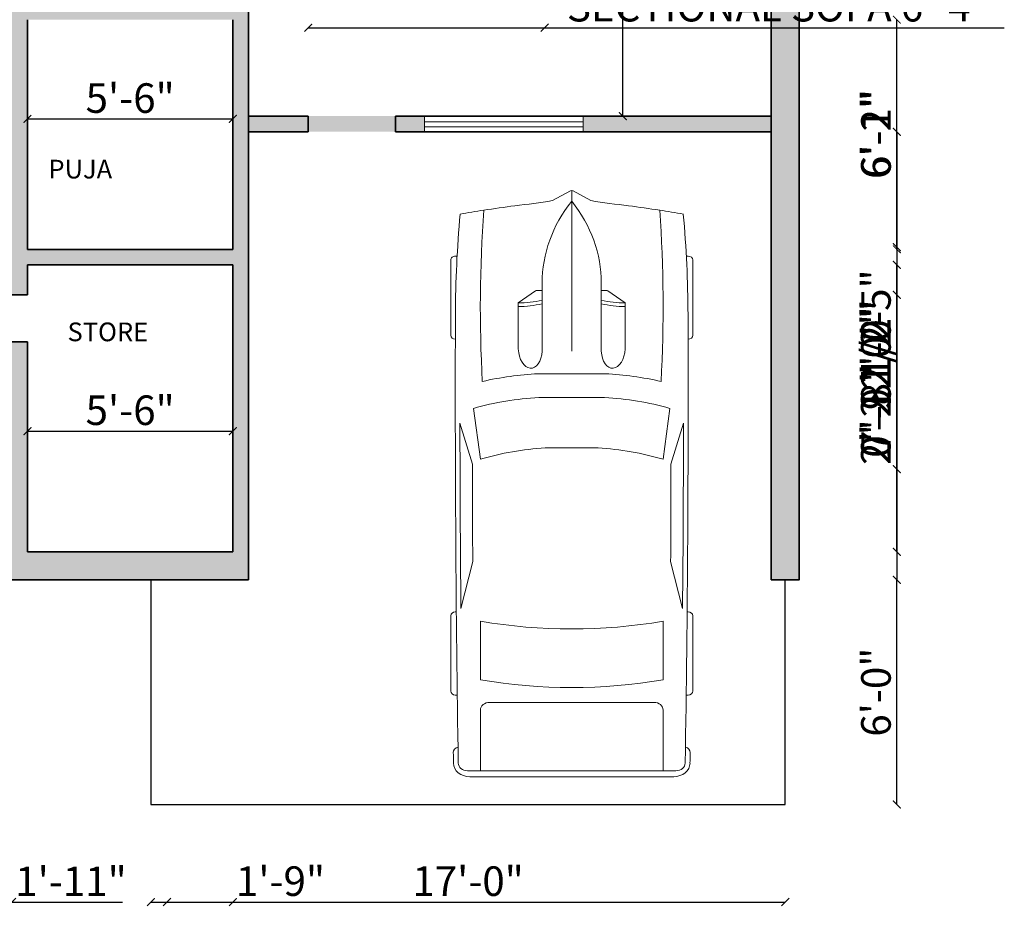
# Model space of a CAD drawing. Units: inches. Extents: x 1704 to 2334, y 1856 to 2559.
# Tile 2 of 10: x 1925 to 2241, y 1863 to 2148. Entities that reach past the tile are written whole.
import ezdxf

# ---------------------------------------------------------------- set-up
doc = ezdxf.new("R2010")
doc.units = ezdxf.units.IN
for name, color, linetype, lineweight in [('A-ANNO-DIMS', 2, 'Continuous', 18), ('A-AREA-IDEN', 7, 'Continuous', 18), ('A-ENTG-VEHC', 9, 'Continuous', 13), ('A-WALL', 7, 'Continuous', 35), ('C-PRKG', 8, 'Continuous', 25), ('WINDOW', 6, 'Continuous', 18)]:
    doc.layers.add(name, color=color, linetype=linetype, lineweight=lineweight)
doc.layers.add('A-WALL-PATT', color=18, linetype='Continuous', lineweight=13, true_color=0x000000)
doc.styles.get("Standard").update_dxf_attribs({"font": 'arial.ttf'})
doc.dimstyles.new('ISO-25', dxfattribs={"dimtxt": 9.5, "dimasz": 2.5, "dimexe": 1.25, "dimexo": 0.625, "dimtad": 1, "dimdec": 0, "dimlunit": 4, "dimtxsty": 'Standard', "dimblk": 'ARCHTICK', "dimcen": 2.5, "dimse1": 1, "dimse2": 1, "dimclrd": 3, "dimadec": 0, "dimazin": 0, "dimtfac": 1, "dimtdec": 0, "dimtmove": 0, "dimatfit": 3, "dimfxl": 1, "dimarcsym": 0})

# ---------------------------------------------------------------- blocks, each defined once
blk = doc.blocks.new('*U6')
for p, q in [((46.55, 38.89), (22.35, 38.89)), ((136.7, 38.89), (160.9, 38.89)), ((21.1, 37.41), (21.1, 36.83)), ((47.8, 37.39), (47.8, 37.41)), ((87.99, 31.87), (74.76, 35.92)), ((134.31, 35.6), (119.29, 31.78)), ((135.45, 37.07), (135.45, 37.41)), ((162.15, 37.41), (162.15, 36.77)), ((186.47, -33.5), (186.47, 33.5)), ((188.4, -32.76), (188.4, 32.76)), ((70.03, 31.54), (86.41, 29.35)), ((138.42, 29.35), (157.25, 29.35)), ((186.47, 29.35), (167.01, 29.35)), ((164.52, 26.39), (164.52, -26.39)), ((32.27, 11.63), (36.13, 17.17)), ((36.13, 17.17), (50.94, 17.17)), ((29.77, 9.51), (51.68, 9.51)), ((32.12, 9.51), (32.12, 11.15)), ((58.92, -10.77), (58.92, 10.77)), ((66.55, -10.53), (66.55, 10.53)), ((186.47, -10.53), (186.47, 10.53)), ((82.74, 8.5), (82.74, -8.5)), ((3.27, 6.13), (0.1, 0.41)), ((0, 0), (51.68, 0)), ((0.1, -0.41), (3.27, -6.13)), ((29.77, -9.51), (51.68, -9.51)), ((32.12, -9.51), (32.12, -11.15)), ((32.27, -11.63), (36.13, -17.17)), ((36.13, -17.17), (50.94, -17.17)), ((86.41, -29.35), (70.03, -31.54)), ((157.25, -29.35), (138.42, -29.35)), ((167.01, -29.35), (186.47, -29.35)), ((87.99, -31.87), (74.76, -35.92)), ((134.31, -35.6), (119.29, -31.78)), ((21.1, -37.41), (21.1, -36.83)), ((47.8, -37.39), (47.8, -37.41)), ((135.45, -37.07), (135.45, -37.41)), ((162.15, -37.41), (162.15, -36.77)), ((46.55, -38.89), (22.35, -38.89)), ((136.7, -38.89), (160.9, -38.89))]:
    blk.add_line(p, q)
for centre, major_axis, ratio, start_param, end_param in [((22.35, 37.41), (0, -1.48), 0.842304, 3.141593, 4.712389), ((46.55, 37.41), (0, 1.48), 0.842304, -1.570796, 0), ((136.7, 37.41), (0, -1.48), 0.842304, 3.141593, 4.712389), ((160.9, 37.41), (0, 1.48), 0.842304, -1.570796, 0), ((180.63, 35.84), (0, 2.22), 0.842304, -0.013017, 1.249894), ((64.48, -10556.36), (0, 10595.31), 0.842304, -0.013397, -0.013017), ((183.98, 32.76), (0, -5.25), 0.842304, 1.570796, 3.128196), ((266.03, -27.52), (0, 313.31), 0.842304, 1.367076, 1.39176), ((41.19, -490.86), (0, 528.23), 0.842304, 0.00281, 0.075598), ((64.48, -10555.62), (0, 10593.03), 0.842304, -0.013397, 0.002797), ((64.48, -10555.62), (0, -10591.55), 0.842304, 3.133765, 3.140441), ((183.98, 33.5), (0, -2.96), 0.842304, 1.570796, 3.128196), ((95.79, -3666.35), (0, -3698.24), 0.842304, 3.134049, 3.144098), ((37.47, -593.96), (0, -623.33), 0.842304, 3.096046, 3.200911), ((134.4, 5.39), (0, -89.78), 0.842304, 4.449482, 4.652344), ((135.29, 5.39), (0, 81.77), 0.842304, 1.245306, 1.50788), ((149.6, 2.8), (0, -79.58), 0.842304, 4.372215, 4.640744), ((17.08, 0), (0, 147.02), 0.842304, 4.511394, 4.913384), ((35.91, 0), (0, 147.02), 0.842304, 4.511394, 4.913384), ((167.01, 26.39), (0, 2.96), 0.842304, 0, 1.570796), ((259.18, -27.52), (0, -305.3), 0.842304, 4.528606, 4.561838), ((-204.49, 52.4), (0, -250.96), 0.842304, 1.385369, 1.434372), ((13.04, 17.01), (0, 27.42), 0.842304, 4.435146, 4.718221), ((14.2, 17.01), (0, 27.42), 0.842304, 4.435146, 4.718221), ((50.79, 13.34), (6.34, -0.36), 0.603834, -1.395552, 1.581315), ((29.77, -46.66), (0, 56.17), 0.842304, 0, 0.590319), ((32.75, 11.15), (0, 0.74), 0.842304, 0.879714, 1.570796), ((0.62, 0), (0, -0.74), 0.842304, 4.131459, 5.293319), ((29.77, 46.66), (0, 56.17), 0.842304, 2.551274, 3.141593), ((-204.49, -52.4), (0, 250.96), 0.842304, -1.434372, -1.385369), ((149.6, -2.8), (0, -79.58), 0.842304, -1.499151, -1.230623), ((32.75, -11.15), (0, -0.74), 0.842304, 4.712389, 5.403472), ((13.04, -17.01), (0, -27.42), 0.842304, 1.564964, 1.848039), ((14.2, -17.01), (0, -27.42), 0.842304, 1.564964, 1.848039), ((134.4, -5.39), (0, -89.78), 0.842304, -1.510751, -1.307889), ((135.29, -5.39), (0, -81.77), 0.842304, -1.50788, -1.245306), ((259.18, 27.52), (0, 305.3), 0.842304, 1.721348, 1.754579), ((266.03, 27.52), (0, 313.31), 0.842304, 1.749832, 1.774517), ((37.47, 593.96), (0, -623.33), 0.842304, -0.059319, 0.045547), ((167.01, -26.39), (0, -2.96), 0.842304, 4.712389, 6.283185), ((95.79, 3666.35), (0, -3698.24), 0.842304, -0.002505, 0.007544), ((183.98, -33.5), (0, 2.96), 0.842304, 3.15499, 4.712389), ((183.98, -32.76), (0, -5.25), 0.842304, 0.013397, 1.570796), ((41.19, 490.86), (0, -528.23), 0.842304, -0.075598, -0.00281), ((22.35, -37.41), (0, 1.48), 0.842304, 1.570796, 3.141593), ((64.48, 10555.62), (0, 10593.03), 0.842304, 3.138796, 3.15499), ((46.55, -37.41), (0, -1.48), 0.842304, 0, 1.570796), ((64.48, 10555.62), (0, -10591.55), 0.842304, 0.001152, 0.007828), ((136.7, -37.41), (0, -1.48), 0.842304, -1.570796, 0), ((160.9, -37.41), (0, 1.48), 0.842304, 3.141593, 4.712389), ((180.63, -35.84), (0, -2.22), 0.842304, -1.249894, 0.013017), ((64.48, 10556.36), (0, 10595.31), 0.842304, 3.15461, 3.15499)]:
    blk.add_ellipse(centre, major_axis=major_axis, ratio=ratio, start_param=start_param, end_param=end_param)
at = {"extrusion": (0, 0, -1)}
blk.add_ellipse((50.79, -13.34), major_axis=(6.34, 0.36), ratio=0.603834, start_param=-1.395552, end_param=1.581315, dxfattribs=at)
blk = doc.blocks.new('_ArchTick')
at = {"color": 0, "linetype": 'ByBlock', "const_width": 0.15}
blk.add_lwpolyline([(-0.5, -0.5), (0.5, 0.5)], dxfattribs=at)
blk = doc.blocks.new('*D18')
at = {"layer": 'A-ANNO-DIMS', "color": 0, "lineweight": -2, "transparency": 16777216}
blk.add_line((1927.01, 2116.15), (1993.01, 2116.15), dxfattribs=at)
at = {"layer": 'Defpoints', "color": 0, "transparency": 16777216}
for p in [(1993.01, 2116.15), (1927.01, 2104.9), (1993.01, 2104.9)]:
    blk.add_point(p, dxfattribs=at)
at = {"layer": 'A-ANNO-DIMS', "color": 0, "lineweight": -2, "transparency": 16777216, "xscale": 2.5, "yscale": 2.5, "zscale": 2.5, "rotation": 180}
blk.add_blockref('_ArchTick', (1927.01, 2116.15), dxfattribs=at)
at = {"layer": 'A-ANNO-DIMS', "color": 0, "lineweight": -2, "transparency": 16777216, "xscale": 2.5, "yscale": 2.5, "zscale": 2.5}
blk.add_blockref('_ArchTick', (1993.01, 2116.15), dxfattribs=at)
at = {"layer": 'A-ANNO-DIMS', "color": 0, "transparency": 16777216, "insert": (1960.01, 2121.62), "char_height": 9.5, "attachment_point": 5}
blk.add_mtext('5\'-6"', dxfattribs=at)
blk = doc.blocks.new('*D19')
at = {"layer": 'A-ANNO-DIMS', "color": 0, "lineweight": -2, "transparency": 16777216}
blk.add_line((1927.01, 2015.83), (1993.01, 2015.83), dxfattribs=at)
at = {"layer": 'Defpoints', "color": 0, "transparency": 16777216}
for p in [(1927.01, 2023.14), (1993.01, 2023.14), (1993.01, 2015.83)]:
    blk.add_point(p, dxfattribs=at)
at = {"layer": 'A-ANNO-DIMS', "color": 0, "lineweight": -2, "transparency": 16777216, "xscale": 2.5, "yscale": 2.5, "zscale": 2.5, "rotation": 180}
blk.add_blockref('_ArchTick', (1927.01, 2015.83), dxfattribs=at)
at = {"layer": 'A-ANNO-DIMS', "color": 0, "lineweight": -2, "transparency": 16777216, "xscale": 2.5, "yscale": 2.5, "zscale": 2.5}
blk.add_blockref('_ArchTick', (1993.01, 2015.83), dxfattribs=at)
at = {"layer": 'A-ANNO-DIMS', "color": 0, "transparency": 16777216, "insert": (1960.01, 2021.31), "char_height": 9.5, "attachment_point": 5}
blk.add_mtext('5\'-6"', dxfattribs=at)
blk = doc.blocks.new('*D21')
at = {"layer": 'A-ANNO-DIMS', "color": 0, "lineweight": -2, "transparency": 16777216}
blk.add_line((2118.31, 2117.04), (2118.31, 2314.04), dxfattribs=at)
at = {"layer": 'Defpoints', "color": 0, "transparency": 16777216}
for p in [(2118.31, 2314.04), (2129.02, 2314.04), (2129.02, 2117.04)]:
    blk.add_point(p, dxfattribs=at)
at = {"layer": 'A-ANNO-DIMS', "color": 0, "lineweight": -2, "transparency": 16777216, "xscale": 2.5, "yscale": 2.5, "zscale": 2.5}
for p, rotation in [((2118.31, 2314.04), 90), ((2118.31, 2117.04), 270)]:
    blk.add_blockref('_ArchTick', p, dxfattribs=dict(at, rotation=rotation))
at = {"layer": 'A-ANNO-DIMS', "color": 0, "transparency": 16777216, "insert": (2112.83, 2215.54), "char_height": 9.5, "attachment_point": 5, "rotation": 90}
blk.add_mtext('16\'-5"', dxfattribs=at)
blk = doc.blocks.new('*D26')
at = {"layer": 'A-ANNO-DIMS', "color": 3, "lineweight": -2, "transparency": 16777216}
for p, q in [((2017.24, 2145.44), (2093.2, 2145.44)), ((2093.2, 2145.44), (2240.89, 2145.44))]:
    blk.add_line(p, q, dxfattribs=at)
at = {"layer": 'Defpoints', "color": 0, "transparency": 16777216}
for p in [(2017.24, 2156.83), (2093.2, 2156.83), (2093.2, 2145.44)]:
    blk.add_point(p, dxfattribs=at)
at = {"layer": 'A-ANNO-DIMS', "color": 3, "lineweight": -2, "transparency": 16777216, "xscale": 2.5, "yscale": 2.5, "zscale": 2.5, "rotation": 180}
blk.add_blockref('_ArchTick', (2017.24, 2145.44), dxfattribs=at)
at = {"layer": 'A-ANNO-DIMS', "color": 3, "lineweight": -2, "transparency": 16777216, "xscale": 2.5, "yscale": 2.5, "zscale": 2.5}
blk.add_blockref('_ArchTick', (2093.2, 2145.44), dxfattribs=at)
at = {"layer": 'A-ANNO-DIMS', "color": 0, "transparency": 16777216, "insert": (2168.29, 2150.98), "char_height": 9.5, "attachment_point": 5}
blk.add_mtext('SECTIONAL SOFA 6\'-4"', dxfattribs=at)
blk = doc.blocks.new('*D34')
at = {"layer": 'A-ANNO-DIMS', "color": 3, "lineweight": -2, "transparency": 16777216}
blk.add_line((2206.36, 1895.85), (2206.36, 1968.04), dxfattribs=at)
at = {"layer": 'Defpoints', "color": 0, "transparency": 16777216}
for p in [(2170.51, 1968.04), (2206.36, 1968.04), (2170.51, 1895.85)]:
    blk.add_point(p, dxfattribs=at)
at = {"layer": 'A-ANNO-DIMS', "color": 3, "lineweight": -2, "transparency": 16777216, "xscale": 2.5, "yscale": 2.5, "zscale": 2.5}
for p, rotation in [((2206.36, 1968.04), 90), ((2206.36, 1895.85), 270)]:
    blk.add_blockref('_ArchTick', p, dxfattribs=dict(at, rotation=rotation))
at = {"layer": 'A-ANNO-DIMS', "color": 0, "transparency": 16777216, "insert": (2200.88, 1931.95), "char_height": 9.5, "attachment_point": 5, "rotation": 90}
blk.add_mtext('6\'-0"', dxfattribs=at)
blk = doc.blocks.new('*D35')
at = {"layer": 'A-ANNO-DIMS', "color": 3, "lineweight": -2, "transparency": 16777216}
blk.add_line((1966.67, 1864.5), (2170.51, 1864.5), dxfattribs=at)
at = {"layer": 'Defpoints', "color": 0, "transparency": 16777216}
for p in [(1966.67, 1895.85), (2170.51, 1895.85), (2170.51, 1864.5)]:
    blk.add_point(p, dxfattribs=at)
at = {"layer": 'A-ANNO-DIMS', "color": 3, "lineweight": -2, "transparency": 16777216, "xscale": 2.5, "yscale": 2.5, "zscale": 2.5, "rotation": 180}
blk.add_blockref('_ArchTick', (1966.67, 1864.5), dxfattribs=at)
at = {"layer": 'A-ANNO-DIMS', "color": 3, "lineweight": -2, "transparency": 16777216, "xscale": 2.5, "yscale": 2.5, "zscale": 2.5}
blk.add_blockref('_ArchTick', (2170.51, 1864.5), dxfattribs=at)
at = {"layer": 'A-ANNO-DIMS', "color": 0, "transparency": 16777216, "insert": (2068.59, 1869.98), "char_height": 9.5, "attachment_point": 5}
blk.add_mtext('17\'-0"', dxfattribs=at)
blk = doc.blocks.new('*D38')
at = {"layer": 'A-ANNO-DIMS', "color": 3, "lineweight": -2, "transparency": 16777216}
blk.add_line((2206.36, 1977.04), (2206.36, 2069.24), dxfattribs=at)
at = {"layer": 'Defpoints', "color": 0, "transparency": 16777216}
for p in [(1927.01, 2069.24), (2206.36, 2069.24), (1927.01, 1977.04)]:
    blk.add_point(p, dxfattribs=at)
at = {"layer": 'A-ANNO-DIMS', "color": 3, "lineweight": -2, "transparency": 16777216, "xscale": 2.5, "yscale": 2.5, "zscale": 2.5}
for p, rotation in [((2206.36, 2069.24), 90), ((2206.36, 1977.04), 270)]:
    blk.add_blockref('_ArchTick', p, dxfattribs=dict(at, rotation=rotation))
at = {"layer": 'A-ANNO-DIMS', "color": 0, "transparency": 16777216, "insert": (2200.88, 2023.14), "char_height": 9.5, "attachment_point": 5, "rotation": 90}
blk.add_mtext('7\'-8"', dxfattribs=at)
blk = doc.blocks.new('*D39')
at = {"layer": 'A-ANNO-DIMS', "color": 3, "lineweight": -2, "transparency": 16777216}
blk.add_line((2206.36, 2074.24), (2206.36, 2148.04), dxfattribs=at)
at = {"layer": 'Defpoints', "color": 0, "transparency": 16777216}
for p in [(1927.01, 2148.04), (2206.36, 2148.04), (1927.01, 2074.24)]:
    blk.add_point(p, dxfattribs=at)
at = {"layer": 'A-ANNO-DIMS', "color": 3, "lineweight": -2, "transparency": 16777216, "xscale": 2.5, "yscale": 2.5, "zscale": 2.5}
for p, rotation in [((2206.36, 2148.04), 90), ((2206.36, 2074.24), 270)]:
    blk.add_blockref('_ArchTick', p, dxfattribs=dict(at, rotation=rotation))
at = {"layer": 'A-ANNO-DIMS', "color": 0, "transparency": 16777216, "insert": (2200.88, 2111.14), "char_height": 9.5, "attachment_point": 5, "rotation": 90}
blk.add_mtext('6\'-2"', dxfattribs=at)
blk = doc.blocks.new('*D42')
at = {"layer": 'A-ANNO-DIMS', "color": 3, "lineweight": -2, "transparency": 16777216}
blk.add_line((2206.36, 2112.04), (2206.36, 1968.04), dxfattribs=at)
at = {"layer": 'Defpoints', "color": 0, "transparency": 16777216}
for p in [(2166.01, 2112.04), (2166.01, 1968.04), (2206.36, 1968.04)]:
    blk.add_point(p, dxfattribs=at)
at = {"layer": 'A-ANNO-DIMS', "color": 3, "lineweight": -2, "transparency": 16777216, "xscale": 2.5, "yscale": 2.5, "zscale": 2.5}
for p, rotation in [((2206.36, 2112.04), 90), ((2206.36, 1968.04), 270)]:
    blk.add_blockref('_ArchTick', p, dxfattribs=dict(at, rotation=rotation))
at = {"layer": 'A-ANNO-DIMS', "color": 0, "transparency": 16777216, "insert": (2200.88, 2040.04), "char_height": 9.5, "attachment_point": 5, "rotation": 90}
blk.add_mtext('12\'-0"', dxfattribs=at)
blk = doc.blocks.new('*D44')
at = {"layer": 'A-ANNO-DIMS', "color": 3, "lineweight": -2, "transparency": 16777216}
for p, q in [((2206.36, 2003.58), (2206.36, 2054.88)), ((2206.36, 1977.04), (2206.36, 2003.58))]:
    blk.add_line(p, q, dxfattribs=at)
at = {"layer": 'Defpoints', "color": 0, "transparency": 16777216}
for p in [(1898.93, 2003.58), (2206.36, 2003.58), (1898.93, 1977.04)]:
    blk.add_point(p, dxfattribs=at)
at = {"layer": 'A-ANNO-DIMS', "color": 3, "lineweight": -2, "transparency": 16777216, "xscale": 2.5, "yscale": 2.5, "zscale": 2.5}
for p, rotation in [((2206.36, 2003.58), 90), ((2206.36, 1977.04), 270)]:
    blk.add_blockref('_ArchTick', p, dxfattribs=dict(at, rotation=rotation))
at = {"layer": 'A-ANNO-DIMS', "color": 0, "transparency": 16777216, "insert": (2200.82, 2030.48), "char_height": 9.5, "attachment_point": 5, "rotation": 90}
blk.add_mtext('2\'-2 1/2"', dxfattribs=at)
blk = doc.blocks.new('*D45')
at = {"layer": 'A-ANNO-DIMS', "color": 3, "lineweight": -2, "transparency": 16777216}
for p, q in [((1898.93, 1864.5), (1922.01, 1864.5)), ((1922.01, 1864.5), (1957.5, 1864.5))]:
    blk.add_line(p, q, dxfattribs=at)
at = {"layer": 'Defpoints', "color": 0, "transparency": 16777216}
for p in [(1898.93, 1977.04), (1922.01, 1977.04), (1922.01, 1864.5)]:
    blk.add_point(p, dxfattribs=at)
at = {"layer": 'A-ANNO-DIMS', "color": 3, "lineweight": -2, "transparency": 16777216, "xscale": 2.5, "yscale": 2.5, "zscale": 2.5, "rotation": 180}
blk.add_blockref('_ArchTick', (1898.93, 1864.5), dxfattribs=at)
at = {"layer": 'A-ANNO-DIMS', "color": 3, "lineweight": -2, "transparency": 16777216, "xscale": 2.5, "yscale": 2.5, "zscale": 2.5}
blk.add_blockref('_ArchTick', (1922.01, 1864.5), dxfattribs=at)
at = {"layer": 'A-ANNO-DIMS', "color": 0, "transparency": 16777216, "insert": (1941, 1869.9), "char_height": 9.5, "attachment_point": 5}
blk.add_mtext('1\'-11"', dxfattribs=at)
blk = doc.blocks.new('*D49')
at = {"layer": 'A-ANNO-DIMS', "color": 3, "lineweight": -2, "transparency": 16777216}
for p, q in [((1998.01, 2539.39), (2017.2, 2539.39)), ((2017.2, 2539.39), (2045.31, 2539.39))]:
    blk.add_line(p, q, dxfattribs=at)
at = {"layer": 'Defpoints', "color": 0, "transparency": 16777216}
for p in [(2017.2, 2539.39), (1998.01, 2117.04), (2017.2, 2117.04)]:
    blk.add_point(p, dxfattribs=at)
at = {"layer": 'A-ANNO-DIMS', "color": 3, "lineweight": -2, "transparency": 16777216, "xscale": 2.5, "yscale": 2.5, "zscale": 2.5, "rotation": 180}
blk.add_blockref('_ArchTick', (1998.01, 2539.39), dxfattribs=at)
at = {"layer": 'A-ANNO-DIMS', "color": 3, "lineweight": -2, "transparency": 16777216, "xscale": 2.5, "yscale": 2.5, "zscale": 2.5}
blk.add_blockref('_ArchTick', (2017.2, 2539.39), dxfattribs=at)
at = {"layer": 'A-ANNO-DIMS', "color": 0, "transparency": 16777216, "insert": (2032.51, 2544.78), "char_height": 9.5, "attachment_point": 5}
blk.add_mtext('1\'-7"', dxfattribs=at)
blk = doc.blocks.new('*D50')
at = {"layer": 'A-ANNO-DIMS', "color": 3, "lineweight": -2, "transparency": 16777216}
blk.add_line((2017.2, 2539.39), (2045.28, 2539.39), dxfattribs=at)
at = {"layer": 'Defpoints', "color": 0, "transparency": 16777216}
for p in [(2045.28, 2539.39), (2017.2, 2117.04), (2045.28, 2117.04)]:
    blk.add_point(p, dxfattribs=at)
at = {"layer": 'A-ANNO-DIMS', "color": 3, "lineweight": -2, "transparency": 16777216, "xscale": 2.5, "yscale": 2.5, "zscale": 2.5, "rotation": 180}
blk.add_blockref('_ArchTick', (2017.2, 2539.39), dxfattribs=at)
at = {"layer": 'A-ANNO-DIMS', "color": 3, "lineweight": -2, "transparency": 16777216, "xscale": 2.5, "yscale": 2.5, "zscale": 2.5}
blk.add_blockref('_ArchTick', (2045.28, 2539.39), dxfattribs=at)
at = {"layer": 'A-ANNO-DIMS', "color": 0, "transparency": 16777216, "insert": (2031.24, 2544.78), "char_height": 9.5, "attachment_point": 5}
blk.add_mtext('2\'-4"', dxfattribs=at)
blk = doc.blocks.new('*D51')
at = {"layer": 'A-ANNO-DIMS', "color": 3, "lineweight": -2, "transparency": 16777216}
for p, q in [((2045.28, 2539.39), (2054.53, 2539.39)), ((2054.53, 2539.39), (2105.67, 2539.39))]:
    blk.add_line(p, q, dxfattribs=at)
at = {"layer": 'Defpoints', "color": 0, "transparency": 16777216}
for p in [(2054.53, 2539.39), (2045.28, 2117.04), (2054.53, 2117.04)]:
    blk.add_point(p, dxfattribs=at)
at = {"layer": 'A-ANNO-DIMS', "color": 3, "lineweight": -2, "transparency": 16777216, "xscale": 2.5, "yscale": 2.5, "zscale": 2.5, "rotation": 180}
blk.add_blockref('_ArchTick', (2045.28, 2539.39), dxfattribs=at)
at = {"layer": 'A-ANNO-DIMS', "color": 3, "lineweight": -2, "transparency": 16777216, "xscale": 2.5, "yscale": 2.5, "zscale": 2.5}
blk.add_blockref('_ArchTick', (2054.53, 2539.39), dxfattribs=at)
at = {"layer": 'A-ANNO-DIMS', "color": 0, "transparency": 16777216, "insert": (2081.35, 2544.93), "char_height": 9.5, "attachment_point": 5}
blk.add_mtext('0\'-9 1/2"', dxfattribs=at)
blk = doc.blocks.new('*D52')
at = {"layer": 'A-ANNO-DIMS', "color": 3, "lineweight": -2, "transparency": 16777216}
blk.add_line((2054.53, 2539.39), (2105.53, 2539.39), dxfattribs=at)
at = {"layer": 'Defpoints', "color": 0, "transparency": 16777216}
for p in [(2105.53, 2539.39), (2054.53, 2117.04), (2105.53, 2117.04)]:
    blk.add_point(p, dxfattribs=at)
at = {"layer": 'A-ANNO-DIMS', "color": 3, "lineweight": -2, "transparency": 16777216, "xscale": 2.5, "yscale": 2.5, "zscale": 2.5, "rotation": 180}
blk.add_blockref('_ArchTick', (2054.53, 2539.39), dxfattribs=at)
at = {"layer": 'A-ANNO-DIMS', "color": 3, "lineweight": -2, "transparency": 16777216, "xscale": 2.5, "yscale": 2.5, "zscale": 2.5}
blk.add_blockref('_ArchTick', (2105.53, 2539.39), dxfattribs=at)
at = {"layer": 'A-ANNO-DIMS', "color": 0, "transparency": 16777216, "insert": (2080.03, 2544.87), "char_height": 9.5, "attachment_point": 5}
blk.add_mtext('4\'-3"', dxfattribs=at)
blk = doc.blocks.new('*D73')
at = {"layer": 'A-ANNO-DIMS', "color": 3, "lineweight": -2, "transparency": 16777216}
for p, q in [((2206.36, 2069.24), (2206.36, 2059.61)), ((2206.36, 2059.61), (2206.36, 2008.47))]:
    blk.add_line(p, q, dxfattribs=at)
at = {"layer": 'Defpoints', "color": 0, "transparency": 16777216}
for p in [(1927.01, 2069.24), (1927.01, 2059.61), (2206.36, 2059.61)]:
    blk.add_point(p, dxfattribs=at)
at = {"layer": 'A-ANNO-DIMS', "color": 3, "lineweight": -2, "transparency": 16777216, "xscale": 2.5, "yscale": 2.5, "zscale": 2.5}
for p, rotation in [((2206.36, 2069.24), 90), ((2206.36, 2059.61), 270)]:
    blk.add_blockref('_ArchTick', p, dxfattribs=dict(at, rotation=rotation))
at = {"layer": 'A-ANNO-DIMS', "color": 0, "transparency": 16777216, "insert": (2200.82, 2032.79), "char_height": 9.5, "attachment_point": 5, "rotation": 90}
blk.add_mtext('0\'-9 1/2"', dxfattribs=at)
blk = doc.blocks.new('*D75')
at = {"layer": 'A-ANNO-DIMS', "color": 3, "lineweight": -2, "transparency": 16777216}
for p, q in [((1971.87, 1864.5), (1993.01, 1864.5)), ((1993.01, 1864.5), (2021.12, 1864.5))]:
    blk.add_line(p, q, dxfattribs=at)
at = {"layer": 'Defpoints', "color": 0, "transparency": 16777216}
for p in [(1971.87, 2148.04), (1993.01, 2148.04), (1993.01, 1864.5)]:
    blk.add_point(p, dxfattribs=at)
at = {"layer": 'A-ANNO-DIMS', "color": 3, "lineweight": -2, "transparency": 16777216, "xscale": 2.5, "yscale": 2.5, "zscale": 2.5, "rotation": 180}
blk.add_blockref('_ArchTick', (1971.87, 1864.5), dxfattribs=at)
at = {"layer": 'A-ANNO-DIMS', "color": 3, "lineweight": -2, "transparency": 16777216, "xscale": 2.5, "yscale": 2.5, "zscale": 2.5}
blk.add_blockref('_ArchTick', (1993.01, 1864.5), dxfattribs=at)
at = {"layer": 'A-ANNO-DIMS', "color": 0, "transparency": 16777216, "insert": (2008.31, 1869.98), "char_height": 9.5, "attachment_point": 5}
blk.add_mtext('1\'-9"', dxfattribs=at)
blk = doc.blocks.new('*D77')
at = {"layer": 'A-ANNO-DIMS', "color": 3, "lineweight": -2, "transparency": 16777216}
for p, q in [((2206.36, 2074.24), (2206.36, 2069.24)), ((2206.36, 2069.24), (2206.36, 2040.24))]:
    blk.add_line(p, q, dxfattribs=at)
at = {"layer": 'Defpoints', "color": 0, "transparency": 16777216}
for p in [(1927.01, 2074.24), (1927.01, 2069.24), (2206.36, 2069.24)]:
    blk.add_point(p, dxfattribs=at)
at = {"layer": 'A-ANNO-DIMS', "color": 3, "lineweight": -2, "transparency": 16777216, "xscale": 2.5, "yscale": 2.5, "zscale": 2.5}
for p, rotation in [((2206.36, 2074.24), 90), ((2206.36, 2069.24), 270)]:
    blk.add_blockref('_ArchTick', p, dxfattribs=dict(at, rotation=rotation))
at = {"layer": 'A-ANNO-DIMS', "color": 0, "transparency": 16777216, "insert": (2200.88, 2053.49), "char_height": 9.5, "attachment_point": 5, "rotation": 90}
blk.add_mtext('0\'-5"', dxfattribs=at)
blk = doc.blocks.new('*D81')
at = {"layer": 'A-ANNO-DIMS', "color": 3, "lineweight": -2, "transparency": 16777216}
blk.add_line((2206.36, 2074.93), (2206.36, 2148.04), dxfattribs=at)
at = {"layer": 'Defpoints', "color": 0, "transparency": 16777216}
for p in [(1796.13, 2148.04), (2206.36, 2148.04), (1790.01, 2074.93)]:
    blk.add_point(p, dxfattribs=at)
at = {"layer": 'A-ANNO-DIMS', "color": 3, "lineweight": -2, "transparency": 16777216, "xscale": 2.5, "yscale": 2.5, "zscale": 2.5}
for p, rotation in [((2206.36, 2148.04), 90), ((2206.36, 2074.93), 270)]:
    blk.add_blockref('_ArchTick', p, dxfattribs=dict(at, rotation=rotation))
at = {"layer": 'A-ANNO-DIMS', "color": 0, "transparency": 16777216, "insert": (2200.88, 2111.48), "char_height": 9.5, "attachment_point": 5, "rotation": 90}
blk.add_mtext('6\'-1"', dxfattribs=at)

msp = doc.modelspace()

# ---------------------------------------------------------------- hatches: boundary and pattern name
at = {"layer": 'A-WALL-PATT'}
h = msp.add_hatch(color=256, dxfattribs=at)
h.dxf.hatch_style = 1
h.paths.add_polyline_path([(1764.01, 2204.96), (1755.01, 2204.96), (1755.01, 2115.31), (1764.01, 2115.31)])
h.paths.add_polyline_path([(1764.01, 2076.84), (1755.01, 2076.84), (1755.01, 1968.04), (1794.77, 1968.04), (1794.77, 1977.04), (1764.01, 1977.04)])
h.paths.add_polyline_path([(1927.01, 1977.04), (1927.01, 2069.24), (1993.01, 2069.24), (1993.01, 1977.04)], flags=16)
h.paths.add_polyline_path([(1927.01, 2074.24), (1927.01, 2148.04), (1993.01, 2148.04), (1993.01, 2074.24)], flags=16)
h.paths.add_polyline_path([(1764.01, 2318.65), (1755.01, 2318.65), (1755.01, 2247.44), (1764.01, 2247.44)])
h.paths.add_polyline_path([(1764.01, 2499.04), (1798.75, 2499.04), (1798.75, 2508.04), (1755.01, 2508.04), (1755.01, 2336.43), (1764.01, 2336.43)])
h.paths.add_polyline_path([(1950.56, 2508.04), (1847.17, 2508.04), (1847.17, 2499.04), (1950.56, 2499.04)])
h.paths.add_polyline_path([(2059.64, 2508.04), (1975.68, 2508.04), (1975.68, 2499.04), (2059.64, 2499.04)])
h.paths.add_polyline_path([(2175.01, 2508.04), (2108.25, 2508.04), (2108.25, 2499.04), (2166.01, 2499.04), (2166.01, 1977.04), (2166.01, 1972.26), (2166.01, 1968.04), (2175.01, 1968.04)])
h.paths.add_polyline_path([(2166.01, 2319.04), (1993.01, 2319.04), (1993.01, 2273.04), (1998.01, 2273.04), (1998.01, 2314.04), (2166.01, 2314.04)])
h.paths.add_polyline_path([(2054.53, 2117.04), (1998.01, 2117.04), (1998.01, 2112.04), (2054.53, 2112.04)])
h.paths.add_polyline_path([(2166.01, 2117.04), (2105.53, 2117.04), (2105.53, 2112.04), (2166.01, 2112.04)])
h.paths.add_polyline_path([(1927.01, 2499.04), (1922.01, 2499.04), (1922.01, 2355.04), (1764.01, 2355.04), (1764.01, 2350.04), (1804.01, 2350.04), (1804.01, 2278.04), (1764.01, 2278.04), (1764.01, 2273.04), (1870.51, 2273.04), (1870.51, 2278.04), (1870.51, 2350.04), (1865.51, 2350.04), (1865.51, 2278.04), (1809.01, 2278.04), (1809.01, 2350.04), (1922.01, 2350.04), (1927.01, 2350.04), (1998.01, 2350.04), (1998.01, 2499.04), (1993.01, 2499.04), (1993.01, 2355.04), (1927.01, 2355.04)])
h.paths.add_polyline_path([(2131.1, 2203.36), (2144.85, 2203.36), (2144.85, 2212.38), (2131.1, 2212.38)], flags=25)
h.paths.add_polyline_path([(2010.94, 2265.21), (2036.85, 2265.21), (2036.85, 2274.23), (2010.94, 2274.23)], flags=9)
h.paths.add_polyline_path([(2010.9, 2274.71), (2056.95, 2274.71), (2056.95, 2284.04), (2010.9, 2284.04)], flags=25)
h.paths.add_polyline_path([(2003.27, 2440.18), (2049.79, 2440.18), (2049.79, 2449.51), (2003.27, 2449.51)], flags=9)
h.paths.add_polyline_path([(1934.96, 2428.22), (1967.48, 2428.22), (1967.48, 2437.55), (1934.96, 2437.55)], flags=25)
h.paths.add_polyline_path([(1778.93, 2466.23), (1827.79, 2466.23), (1827.79, 2475.56), (1778.93, 2475.56)], flags=25)
h.paths.add_polyline_path([(1938.32, 2043.05), (1970.37, 2043.05), (1970.37, 2052.39), (1938.32, 2052.39)], flags=8)
h.paths.add_polyline_path([(1932.21, 2095.38), (1956.75, 2095.38), (1956.75, 2104.56), (1932.21, 2104.56)], flags=8)
h.paths.add_polyline_path([(1888.97, 2148.04), (1888.97, 2153.04), (1764.01, 2153.04), (1764.01, 2148.04)])
h.paths.add_polyline_path([(1922.01, 2059.61), (1927.01, 2059.61), (1927.01, 2044.47), (1922.01, 2044.47), (1922.01, 1977.04), (1857.04, 1977.04), (1857.04, 1968.04), (1998.01, 1968.04), (1998.01, 1977.04), (1998.01, 2153.04), (1916.93, 2153.04), (1916.93, 2148.04), (1922.01, 2148.04)])

# ---------------------------------------------------------------- linework, layer by layer
at = {"layer": 'A-WALL'}
for p, q in [((2166.01, 2499.04), (2166.01, 1977.04)), ((1998.01, 1977.04), (1998.01, 2153.04)), ((1927.01, 2074.24), (1927.01, 2148.04)), ((1993.01, 2074.24), (1993.01, 2148.04)), ((1998.01, 2117.04), (2017.2, 2117.04)), ((2017.2, 2117.04), (2017.2, 2112.04)), ((2045.28, 2117.04), (2045.28, 2112.04)), ((2045.28, 2117.04), (2166.01, 2117.04)), ((1998.01, 2112.04), (2017.2, 2112.04)), ((2045.28, 2112.04), (2166.01, 2112.04)), ((1927.01, 2074.24), (1993.01, 2074.24)), ((1927.01, 2069.24), (1993.01, 2069.24)), ((1927.01, 2059.61), (1927.01, 2069.24)), ((1993.01, 1977.04), (1993.01, 2069.24)), ((1927.01, 2059.61), (1922.01, 2059.61)), ((1927.01, 2044.47), (1922.01, 2044.47)), ((1927.01, 1977.04), (1927.01, 2044.47)), ((1993.01, 1977.04), (1927.01, 1977.04)), ((1998.01, 1977.04), (1998.01, 1968.04)), ((2166.01, 1977.04), (2166.01, 1972.26)), ((2166.01, 1972.26), (2166.01, 1968.04))]:
    msp.add_line(p, q, dxfattribs=at)
msp.add_lwpolyline([(1998.01, 1968.04), (1755.01, 1968.04), (1755.01, 2508.04), (2175.01, 2508.04), (2175.01, 1968.04), (2166.01, 1968.04)], dxfattribs=at)
at = {"layer": 'C-PRKG'}
for p, q in [((1966.67, 1968.04), (1966.67, 1895.85)), ((2170.51, 1895.85), (2170.51, 1968.04)), ((1966.67, 1895.85), (2170.51, 1895.85))]:
    msp.add_line(p, q, dxfattribs=at)
at = {"layer": 'WINDOW'}
for p, q in [((2054.53, 2117.04), (2054.53, 2112.04)), ((2105.53, 2117.04), (2054.53, 2117.04)), ((2105.53, 2112.04), (2105.53, 2117.04)), ((2105.53, 2115.25), (2054.53, 2115.25)), ((2105.53, 2113.62), (2054.53, 2113.62)), ((2054.53, 2112.04), (2105.53, 2112.04))]:
    msp.add_line(p, q, dxfattribs=at)

# ---------------------------------------------------------------- block references
at = {"layer": 'A-ENTG-VEHC', "rotation": 270}
msp.add_blockref('*U6', (2101.89, 2093.17), dxfattribs=at)

# ---------------------------------------------------------------- texts
at = {"layer": 'A-AREA-IDEN'}
for s, p in [('PUJA', (1933.74, 2097.01)), ('STORE', (1939.87, 2044.71))]:
    msp.add_text(s, height=6.013, dxfattribs=at).set_placement(p)

# ---------------------------------------------------------------- dimensions: what is measured, and where the dimension line sits
at = {"layer": 'A-ANNO-DIMS'}
for base, p1, p2, override, picture, middle in [((2054.5307, 2539.3895), (2045.2758, 2117.0395), (2054.5307, 2117.0395), {"dimdec": 1, "dimlfac": 1, "dimrnd": 0, "dimzin": 1, "dimdsep": 46, "dimlunit": 4, "dimfrac": 2}, '*D51', (2081.3506, 2544.9265)), ((2017.2, 2539.39), (1998.01, 2117.04), (2017.2, 2117.04), {"dimdec": 1, "dimlfac": 1, "dimrnd": 0, "dimzin": 1, "dimdsep": 46, "dimlunit": 4, "dimfrac": 2}, '*D49', (2032.51, 2544.78)), ((2045.28, 2539.39), (2017.2, 2117.04), (2045.28, 2117.04), {"dimdec": 1, "dimlfac": 1, "dimrnd": 0, "dimzin": 1, "dimdsep": 46, "dimlunit": 4, "dimfrac": 2}, '*D50', (2031.24, 2544.78)), ((2105.53, 2539.39), (2054.53, 2117.04), (2105.53, 2117.04), {"dimdec": 1, "dimlfac": 1, "dimrnd": 0, "dimzin": 1, "dimdsep": 46, "dimlunit": 4, "dimfrac": 2}, '*D52', (2080.03, 2544.87)), ((1993.01, 1864.5), (1971.87, 2148.04), (1993.01, 2148.04), {"dimdec": 1, "dimlfac": 1, "dimrnd": 0, "dimzin": 1, "dimdsep": 46, "dimlunit": 4, "dimfrac": 2}, '*D75', (2008.31, 1869.98)), ((1993.01, 2116.15), (1927.01, 2104.9), (1993.01, 2104.9), {"dimclrd": 0, "dimclre": 0, "dimclrt": 0}, '*D18', (1960.01, 2121.62)), ((1993.01, 2015.83), (1927.01, 2023.14), (1993.01, 2023.14), {"dimclrd": 0, "dimclre": 0, "dimclrt": 0}, '*D19', (1960.01, 2021.31)), ((1922.01, 1864.5), (1898.93, 1977.04), (1922.01, 1977.04), {"dimdec": 1, "dimlfac": 1, "dimrnd": 0, "dimzin": 1, "dimdsep": 46, "dimlunit": 4, "dimfrac": 2}, '*D45', (1941, 1869.9)), ((2170.51, 1864.5), (1966.67, 1895.85), (2170.51, 1895.85), {"dimdec": 1, "dimlfac": 1, "dimrnd": 0, "dimzin": 1, "dimdsep": 46, "dimlunit": 4, "dimfrac": 2}, '*D35', (2068.59, 1869.98))]:
    dim = msp.add_linear_dim(base=base, p1=p1, p2=p2, dimstyle='ISO-25', override=override, dxfattribs=at)
    dim.commit()
    dim.dimension.update_dxf_attribs({"geometry": picture, "text_midpoint": middle})
for base, p1, p2, override, picture, middle in [((2118.31, 2314.04), (2129.02, 2117.04), (2129.02, 2314.04), {"dimclrd": 0, "dimclre": 0, "dimclrt": 0}, '*D21', (2112.83, 2215.54)), ((2206.36, 2148.04), (1790.01, 2074.93), (1796.13, 2148.04), {"dimdec": 1, "dimlfac": 1, "dimrnd": 0, "dimzin": 1, "dimdsep": 46, "dimlunit": 4, "dimfrac": 2}, '*D81', (2200.88, 2111.48)), ((2206.36, 2148.04), (1927.01, 2074.24), (1927.01, 2148.04), {"dimdec": 1, "dimlfac": 1, "dimrnd": 0, "dimzin": 1, "dimdsep": 46, "dimlunit": 4, "dimfrac": 2}, '*D39', (2200.88, 2111.14)), ((2206.36, 1968.04), (2166.01, 2112.04), (2166.01, 1968.04), {"dimdec": 1, "dimlfac": 1, "dimrnd": 0, "dimzin": 1, "dimdsep": 46, "dimlunit": 4, "dimfrac": 2}, '*D42', (2200.88, 2040.04)), ((2206.36, 2069.24), (1927.01, 2074.24), (1927.01, 2069.24), {"dimdec": 1, "dimlfac": 1, "dimrnd": 0, "dimzin": 1, "dimdsep": 46, "dimlunit": 4, "dimfrac": 2}, '*D77', (2200.88, 2053.49)), ((2206.36, 2069.24), (1927.01, 1977.04), (1927.01, 2069.24), {"dimdec": 1, "dimlfac": 1, "dimrnd": 0, "dimzin": 1, "dimdsep": 46, "dimlunit": 4, "dimfrac": 2}, '*D38', (2200.88, 2023.14)), ((2206.36, 2059.61), (1927.01, 2069.24), (1927.01, 2059.61), {"dimdec": 1, "dimlfac": 1, "dimrnd": 0, "dimzin": 1, "dimdsep": 46, "dimlunit": 4, "dimfrac": 2}, '*D73', (2200.82, 2032.79)), ((2206.36, 2003.58), (1898.93, 1977.04), (1898.93, 2003.58), {"dimdec": 1, "dimlfac": 1, "dimrnd": 0, "dimzin": 1, "dimdsep": 46, "dimlunit": 4, "dimfrac": 2}, '*D44', (2200.82, 2030.48)), ((2206.36, 1968.04), (2170.51, 1895.85), (2170.51, 1968.04), {"dimdec": 1, "dimlfac": 1, "dimrnd": 0, "dimzin": 1, "dimdsep": 46, "dimlunit": 4, "dimfrac": 2}, '*D34', (2200.88, 1931.95))]:
    dim = msp.add_linear_dim(base=base, p1=p1, p2=p2, angle=90, dimstyle='ISO-25', override=override, dxfattribs=at)
    dim.commit()
    dim.dimension.update_dxf_attribs({"geometry": picture, "text_midpoint": middle})
dim = msp.add_linear_dim(base=(2093.2, 2145.44), p1=(2017.24, 2156.83), p2=(2093.2, 2156.83), text='SECTIONAL SOFA <>', dimstyle='ISO-25', override={"dimdec": 1, "dimlfac": 1, "dimrnd": 0, "dimzin": 1, "dimdsep": 46, "dimlunit": 4, "dimfrac": 2}, dxfattribs=at)
dim.commit()
dim.dimension.update_dxf_attribs({"geometry": '*D26', "text_midpoint": (2168.29, 2150.98)})

doc.saveas('drawing.dxf')
